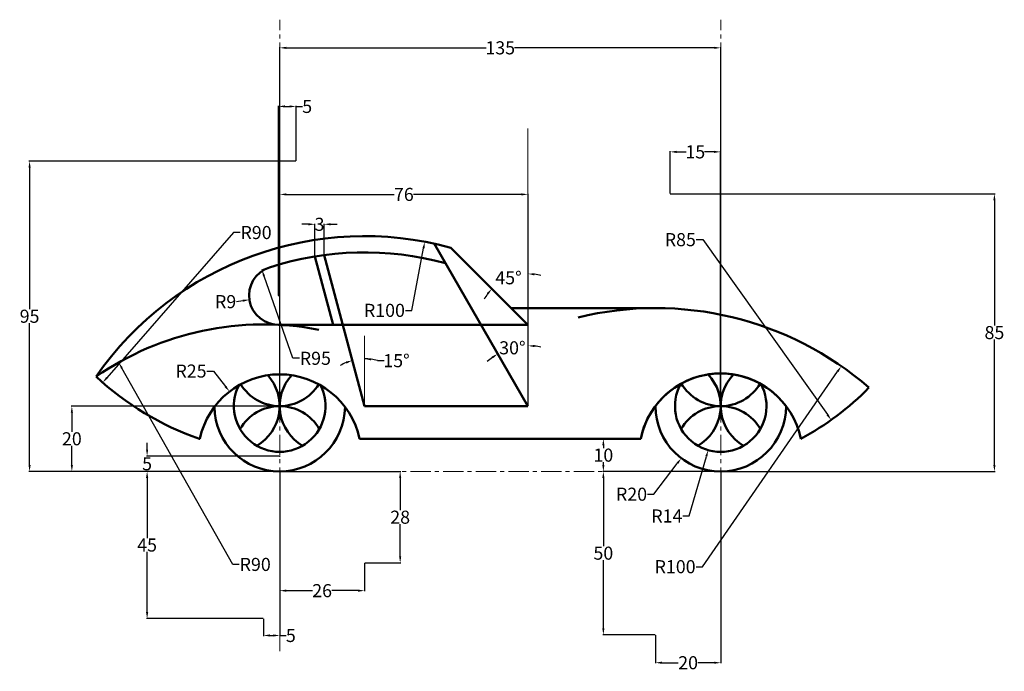
# Model space of a CAD drawing. Units: millimetres. Extents: x -64 to 541, y -54 to 145.
# Tile 1 of 2: x -64 to 238, y -54 to 145. Entities that reach past the tile are written whole.
import ezdxf

# ---------------------------------------------------------------- set-up
doc = ezdxf.new("R2010")
doc.units = ezdxf.units.MM
doc.header["$MEASUREMENT"] = 0
doc.linetypes.add('CENTER', pattern=[2, 1.25, -0.25, 0.25, -0.25])
for name, color, linetype, lineweight in [('M-CNTR', 4, 'CENTER', 18), ('M-CONS', 8, 'Continuous', 13), ('M-DIMS', 2, 'Continuous', 25), ('M-OUTL', 7, 'Continuous', 50)]:
    doc.layers.add(name, color=color, linetype=linetype, lineweight=lineweight)
doc.styles.get("Standard").update_dxf_attribs({"font": 'arial.ttf'})
doc.dimstyles.get("Standard").update_dxf_attribs({"dimtxt": 4, "dimasz": 2, "dimexe": 0.18, "dimexo": 0.0625, "dimgap": 0.09, "dimtad": 0, "dimtih": 1, "dimtoh": 1, "dimdec": 0, "dimzin": 0, "dimdsep": 46, "dimtxsty": 'Standard', "dimcen": 0.09, "dimadec": 0, "dimazin": 0, "dimtfac": 1, "dimtdec": 0, "dimtofl": 0, "dimtmove": 0, "dimatfit": 3, "dimfxl": 1, "dimtolj": 1, "dimtzin": 0, "dimarcsym": 0})

# ---------------------------------------------------------------- blocks, each defined once
blk = doc.blocks.new('*D2')
at = {"layer": 'Defpoints', "color": 0, "transparency": 16777216}
for p in [(15.99, 6.84), (41.96, -21.13), (41.96, -29.63)]:
    blk.add_point(p, dxfattribs=at)
at = {"layer": 'M-DIMS', "color": 0, "lineweight": -2, "transparency": 16777216}
for p, q in [((15.99, 6.78), (15.99, -29.81)), ((41.96, -21.2), (41.96, -29.81)), ((17.99, -29.63), (25.98, -29.63)), ((39.96, -29.63), (31.96, -29.63))]:
    blk.add_line(p, q, dxfattribs=at)
at = {"layer": 'M-DIMS', "color": 0, "transparency": 16777216}
for points in [[(17.99, -29.3), (17.99, -29.97), (15.99, -29.63)], [(39.96, -29.3), (39.96, -29.97), (41.96, -29.63)]]:
    blk.add_solid(points, dxfattribs=at)
at = {"layer": 'M-DIMS', "color": 0, "transparency": 16777216, "insert": (28.97, -29.63), "char_height": 4, "attachment_point": 5}
blk.add_mtext('\\A1;26', dxfattribs=at)
blk = doc.blocks.new('*D3')
at = {"layer": 'Defpoints', "color": 0, "transparency": 16777216}
for p in [(15.99, 6.84), (41.96, -21.13), (52.86, -21.13)]:
    blk.add_point(p, dxfattribs=at)
at = {"layer": 'M-DIMS', "color": 0, "lineweight": -2, "transparency": 16777216}
for p, q in [((16.05, 6.84), (53.04, 6.84)), ((52.86, 4.84), (52.86, -5.02)), ((52.86, -19.13), (52.86, -9.28)), ((42.02, -21.13), (53.04, -21.13))]:
    blk.add_line(p, q, dxfattribs=at)
at = {"layer": 'M-DIMS', "color": 0, "transparency": 16777216}
for points in [[(52.53, 4.84), (53.19, 4.84), (52.86, 6.84)], [(52.53, -19.13), (53.19, -19.13), (52.86, -21.13)]]:
    blk.add_solid(points, dxfattribs=at)
at = {"layer": 'M-DIMS', "color": 0, "transparency": 16777216, "insert": (52.86, -7.15), "char_height": 4, "attachment_point": 5}
blk.add_mtext('\\A1;28', dxfattribs=at)
blk = doc.blocks.new('*D4')
at = {"layer": 'Defpoints', "color": 0, "transparency": 16777216}
for p in [(15.99, 6.84), (10.99, -38.16), (15.99, -43.35)]:
    blk.add_point(p, dxfattribs=at)
at = {"layer": 'M-DIMS', "color": 0, "lineweight": -2, "transparency": 16777216}
for p, q in [((15.99, 6.78), (15.99, -43.53)), ((10.99, -38.22), (10.99, -43.53)), ((12.99, -43.35), (13.99, -43.35)), ((15.99, -43.35), (17.99, -43.35))]:
    blk.add_line(p, q, dxfattribs=at)
at = {"layer": 'M-DIMS', "color": 0, "transparency": 16777216}
for points in [[(12.99, -43.01), (12.99, -43.68), (10.99, -43.35)], [(13.99, -43.01), (13.99, -43.68), (15.99, -43.35)]]:
    blk.add_solid(points, dxfattribs=at)
at = {"layer": 'M-DIMS', "color": 0, "transparency": 16777216, "insert": (19.4, -43.35), "char_height": 4, "attachment_point": 5}
blk.add_mtext('\\A1;5', dxfattribs=at)
blk = doc.blocks.new('*D5')
at = {"layer": 'Defpoints', "color": 0, "transparency": 16777216}
for p in [(-24.6, 6.84), (15.99, 6.84), (10.99, -38.16)]:
    blk.add_point(p, dxfattribs=at)
at = {"layer": 'M-DIMS', "color": 0, "lineweight": -2, "transparency": 16777216}
for p, q in [((15.92, 6.84), (-24.78, 6.84)), ((-24.6, 4.84), (-24.6, -13.54)), ((-24.6, -36.16), (-24.6, -17.79)), ((10.92, -38.16), (-24.78, -38.16))]:
    blk.add_line(p, q, dxfattribs=at)
at = {"layer": 'M-DIMS', "color": 0, "transparency": 16777216}
for points in [[(-24.93, 4.84), (-24.26, 4.84), (-24.6, 6.84)], [(-24.93, -36.16), (-24.26, -36.16), (-24.6, -38.16)]]:
    blk.add_solid(points, dxfattribs=at)
at = {"layer": 'M-DIMS', "color": 0, "transparency": 16777216, "insert": (-24.6, -15.66), "char_height": 4, "attachment_point": 5}
blk.add_mtext('\\A1;45', dxfattribs=at)
blk = doc.blocks.new('*D6')
at = {"layer": 'Defpoints', "color": 0, "transparency": 16777216}
for p in [(-47.63, 26.84), (15.99, 26.84), (15.99, 6.84)]:
    blk.add_point(p, dxfattribs=at)
at = {"layer": 'M-DIMS', "color": 0, "lineweight": -2, "transparency": 16777216}
for p, q in [((15.92, 26.84), (-47.81, 26.84)), ((-47.63, 24.84), (-47.63, 18.97)), ((-47.63, 8.84), (-47.63, 14.71)), ((15.92, 6.84), (-47.81, 6.84))]:
    blk.add_line(p, q, dxfattribs=at)
at = {"layer": 'M-DIMS', "color": 0, "transparency": 16777216}
for points in [[(-47.96, 24.84), (-47.29, 24.84), (-47.63, 26.84)], [(-47.96, 8.84), (-47.29, 8.84), (-47.63, 6.84)]]:
    blk.add_solid(points, dxfattribs=at)
at = {"layer": 'M-DIMS', "color": 0, "transparency": 16777216, "insert": (-47.63, 16.84), "char_height": 4, "attachment_point": 5}
blk.add_mtext('\\A1;20', dxfattribs=at)
blk = doc.blocks.new('*D7')
at = {"layer": 'Defpoints', "color": 0, "transparency": 16777216}
for p in [(-33.29, 40.19), (10.99, -38.16)]:
    blk.add_point(p, dxfattribs=at)
at = {"layer": 'M-DIMS', "color": 0, "lineweight": -2, "transparency": 16777216}
for p, q in [((1.63, -21.6), (-32.31, 38.45)), ((3.63, -21.6), (1.63, -21.6))]:
    blk.add_line(p, q, dxfattribs=at)
at = {"layer": 'M-DIMS', "color": 0, "transparency": 16777216}
blk.add_solid([(-32.02, 38.62), (-32.6, 38.29), (-33.29, 40.19)], dxfattribs=at)
at = {"layer": 'M-DIMS', "color": 0, "transparency": 16777216, "insert": (8.49, -21.6), "char_height": 4, "attachment_point": 5}
blk.add_mtext('\\A1;R90', dxfattribs=at)
blk = doc.blocks.new('*D8')
at = {"layer": 'Defpoints', "color": 0, "transparency": 16777216}
for p in [(0.62, 31.28), (15.99, 11.56)]:
    blk.add_point(p, dxfattribs=at)
at = {"layer": 'M-DIMS', "color": 0, "lineweight": -2, "transparency": 16777216}
for p, q in [((-6.28, 37.57), (-4.28, 37.57)), ((-4.28, 37.57), (-0.61, 32.86)), ((15.9, 11.56), (16.08, 11.56)), ((15.99, 11.47), (15.99, 11.65))]:
    blk.add_line(p, q, dxfattribs=at)
at = {"layer": 'M-DIMS', "color": 0, "transparency": 16777216}
blk.add_solid([(-0.34, 33.06), (-0.87, 32.65), (0.62, 31.28)], dxfattribs=at)
at = {"layer": 'M-DIMS', "color": 0, "transparency": 16777216, "insert": (-11.16, 37.57), "char_height": 4, "attachment_point": 5}
blk.add_mtext('\\A1;R25', dxfattribs=at)
blk = doc.blocks.new('*D9')
at = {"layer": 'Defpoints', "color": 0, "transparency": 16777216}
for p in [(10.54, 68.52), (41.96, -21.13)]:
    blk.add_point(p, dxfattribs=at)
at = {"layer": 'M-DIMS', "color": 0, "lineweight": -2, "transparency": 16777216}
for p, q in [((20.02, 41.47), (11.2, 66.63)), ((22.02, 41.47), (20.02, 41.47))]:
    blk.add_line(p, q, dxfattribs=at)
blk.add_arc((41.96, -21.13), 95, 107.8791, 109.4219, dxfattribs=at)
at = {"layer": 'M-DIMS', "color": 0, "transparency": 16777216}
blk.add_solid([(11.51, 66.74), (10.88, 66.52), (10.54, 68.52)], dxfattribs=at)
at = {"layer": 'M-DIMS', "color": 0, "transparency": 16777216, "insert": (26.9, 41.47), "char_height": 4, "attachment_point": 5}
blk.add_mtext('\\A1;R95', dxfattribs=at)
blk = doc.blocks.new('*D10')
at = {"layer": 'Defpoints', "color": 0, "transparency": 16777216}
for p in [(60.39, 77.15), (41.96, -21.13)]:
    blk.add_point(p, dxfattribs=at)
at = {"layer": 'M-DIMS', "color": 0, "lineweight": -2, "transparency": 16777216}
for p, q in [((56.45, 56.14), (60.02, 75.19)), ((54.45, 56.14), (56.45, 56.14))]:
    blk.add_line(p, q, dxfattribs=at)
at = {"layer": 'M-DIMS', "color": 0, "transparency": 16777216}
blk.add_solid([(59.7, 75.25), (60.35, 75.12), (60.39, 77.15)], dxfattribs=at)
at = {"layer": 'M-DIMS', "color": 0, "transparency": 16777216, "insert": (48.04, 56.14), "char_height": 4, "attachment_point": 5}
blk.add_mtext('\\A1;R100', dxfattribs=at)
blk = doc.blocks.new('*D11')
at = {"layer": 'Defpoints', "color": 0, "transparency": 16777216}
for p in [(20.99, 101.84), (-38.19, 34.03)]:
    blk.add_point(p, dxfattribs=at)
at = {"layer": 'M-DIMS', "color": 0, "lineweight": -2, "transparency": 16777216}
for p, q in [((1.89, 79.95), (-36.88, 35.54)), ((3.89, 79.95), (1.89, 79.95))]:
    blk.add_line(p, q, dxfattribs=at)
at = {"layer": 'M-DIMS', "color": 0, "transparency": 16777216}
blk.add_solid([(-37.13, 35.76), (-36.63, 35.32), (-38.19, 34.03)], dxfattribs=at)
at = {"layer": 'M-DIMS', "color": 0, "transparency": 16777216, "insert": (8.75, 79.95), "char_height": 4, "attachment_point": 5}
blk.add_mtext('\\A1;R90', dxfattribs=at)
blk = doc.blocks.new('*D12')
at = {"layer": 'Defpoints', "color": 0, "transparency": 16777216}
for p in [(91.99, 91.62), (15.99, 26.84), (91.99, 26.84)]:
    blk.add_point(p, dxfattribs=at)
at = {"layer": 'M-DIMS', "color": 0, "lineweight": -2, "transparency": 16777216}
for p, q in [((15.99, 26.9), (15.99, 91.8)), ((17.99, 91.62), (51.05, 91.62)), ((89.99, 91.62), (56.92, 91.62)), ((91.99, 26.9), (91.99, 91.8))]:
    blk.add_line(p, q, dxfattribs=at)
at = {"layer": 'M-DIMS', "color": 0, "transparency": 16777216}
for points in [[(17.99, 91.95), (17.99, 91.29), (15.99, 91.62)], [(89.99, 91.95), (89.99, 91.29), (91.99, 91.62)]]:
    blk.add_solid(points, dxfattribs=at)
at = {"layer": 'M-DIMS', "color": 0, "transparency": 16777216, "insert": (53.99, 91.62), "char_height": 4, "attachment_point": 5}
blk.add_mtext('\\A1;76', dxfattribs=at)
blk = doc.blocks.new('*D13')
at = {"layer": 'Defpoints', "color": 0, "transparency": 16777216}
for p in [(29.57, 82.48), (26.76, 72.64), (29.57, 73.05)]:
    blk.add_point(p, dxfattribs=at)
at = {"layer": 'M-DIMS', "color": 0, "lineweight": -2, "transparency": 16777216}
for p, q in [((24.76, 82.48), (22.76, 82.48)), ((26.76, 72.71), (26.76, 82.66)), ((29.57, 73.12), (29.57, 82.66)), ((31.57, 82.48), (33.57, 82.48))]:
    blk.add_line(p, q, dxfattribs=at)
at = {"layer": 'M-DIMS', "color": 0, "transparency": 16777216}
for points in [[(24.76, 82.82), (24.76, 82.15), (26.76, 82.48)], [(31.57, 82.82), (31.57, 82.15), (29.57, 82.48)]]:
    blk.add_solid(points, dxfattribs=at)
at = {"layer": 'M-DIMS', "color": 0, "transparency": 16777216, "insert": (28.17, 82.48), "char_height": 4, "attachment_point": 5}
blk.add_mtext('\\A1;3', dxfattribs=at)
blk = doc.blocks.new('*D14')
at = {"layer": 'Defpoints', "color": 0, "transparency": 16777216}
for p in [(15.61, 60.73), (6.71, 59.4)]:
    blk.add_point(p, dxfattribs=at)
at = {"layer": 'M-DIMS', "color": 0, "lineweight": -2, "transparency": 16777216}
for p, q in [((15.52, 60.73), (15.7, 60.73)), ((15.61, 60.64), (15.61, 60.82)), ((2.75, 58.81), (4.73, 59.11))]:
    blk.add_line(p, q, dxfattribs=at)
at = {"layer": 'M-DIMS', "color": 0, "transparency": 16777216}
blk.add_solid([(4.68, 59.44), (4.78, 58.78), (6.71, 59.4)], dxfattribs=at)
at = {"layer": 'M-DIMS', "color": 0, "transparency": 16777216, "insert": (-0.57, 58.81), "char_height": 4, "attachment_point": 5}
blk.add_mtext('\\A1;R9', dxfattribs=at)
blk = doc.blocks.new('*D15')
at = {"layer": 'Defpoints', "color": 0, "transparency": 16777216}
for p in [(20.99, 118.54), (20.99, 101.84), (15.61, 60.73)]:
    blk.add_point(p, dxfattribs=at)
at = {"layer": 'M-DIMS', "color": 0, "lineweight": -2, "transparency": 16777216}
for p, q in [((15.61, 60.79), (15.61, 118.72)), ((17.61, 118.54), (18.99, 118.54)), ((20.99, 101.9), (20.99, 118.72)), ((20.99, 118.54), (22.99, 118.54))]:
    blk.add_line(p, q, dxfattribs=at)
at = {"layer": 'M-DIMS', "color": 0, "transparency": 16777216}
for points in [[(17.61, 118.87), (17.61, 118.21), (15.61, 118.54)], [(18.99, 118.87), (18.99, 118.21), (20.99, 118.54)]]:
    blk.add_solid(points, dxfattribs=at)
at = {"layer": 'M-DIMS', "color": 0, "transparency": 16777216, "insert": (24.4, 118.54), "char_height": 4, "attachment_point": 5}
blk.add_mtext('\\A1;5', dxfattribs=at)
blk = doc.blocks.new('*D16')
at = {"layer": 'Defpoints', "color": 0, "transparency": 16777216}
for p in [(-60.57, 101.84), (20.99, 101.84), (15.99, 6.84)]:
    blk.add_point(p, dxfattribs=at)
at = {"layer": 'M-DIMS', "color": 0, "lineweight": -2, "transparency": 16777216}
for p, q in [((20.92, 101.84), (-60.75, 101.84)), ((-60.57, 99.84), (-60.57, 56.47)), ((-60.57, 8.84), (-60.57, 52.21)), ((15.92, 6.84), (-60.75, 6.84))]:
    blk.add_line(p, q, dxfattribs=at)
at = {"layer": 'M-DIMS', "color": 0, "transparency": 16777216}
for points in [[(-60.9, 99.84), (-60.24, 99.84), (-60.57, 101.84)], [(-60.9, 8.84), (-60.24, 8.84), (-60.57, 6.84)]]:
    blk.add_solid(points, dxfattribs=at)
at = {"layer": 'M-DIMS', "color": 0, "transparency": 16777216, "insert": (-60.57, 54.34), "char_height": 4, "attachment_point": 5}
blk.add_mtext('\\A1;95', dxfattribs=at)
blk = doc.blocks.new('*D17')
at = {"layer": 'Defpoints', "color": 0, "transparency": 16777216}
for p in [(150.99, 136.47), (15.99, 26.84), (150.99, 26.84)]:
    blk.add_point(p, dxfattribs=at)
at = {"layer": 'M-DIMS', "color": 0, "lineweight": -2, "transparency": 16777216}
for p, q in [((15.99, 26.9), (15.99, 136.65)), ((17.99, 136.47), (79.15, 136.47)), ((148.99, 136.47), (87.82, 136.47)), ((150.99, 26.9), (150.99, 136.65))]:
    blk.add_line(p, q, dxfattribs=at)
at = {"layer": 'M-DIMS', "color": 0, "transparency": 16777216}
for points in [[(17.99, 136.8), (17.99, 136.14), (15.99, 136.47)], [(148.99, 136.8), (148.99, 136.14), (150.99, 136.47)]]:
    blk.add_solid(points, dxfattribs=at)
at = {"layer": 'M-DIMS', "color": 0, "transparency": 16777216, "insert": (83.49, 136.47), "char_height": 4, "attachment_point": 5}
blk.add_mtext('\\A1;135', dxfattribs=at)
blk = doc.blocks.new('*D18')
at = {"layer": 'Defpoints', "color": 0, "transparency": 16777216}
for p in [(126.49, 16.84), (115.05, 6.84), (150.99, 6.84)]:
    blk.add_point(p, dxfattribs=at)
at = {"layer": 'M-DIMS', "color": 0, "lineweight": -2, "transparency": 16777216}
for p, q in [((126.43, 16.84), (114.87, 16.84)), ((115.05, 14.84), (115.05, 13.97)), ((115.05, 8.84), (115.05, 9.71)), ((150.92, 6.84), (114.87, 6.84))]:
    blk.add_line(p, q, dxfattribs=at)
at = {"layer": 'M-DIMS', "color": 0, "transparency": 16777216}
for points in [[(114.72, 14.84), (115.39, 14.84), (115.05, 16.84)], [(114.72, 8.84), (115.39, 8.84), (115.05, 6.84)]]:
    blk.add_solid(points, dxfattribs=at)
at = {"layer": 'M-DIMS', "color": 0, "transparency": 16777216, "insert": (115.05, 11.84), "char_height": 4, "attachment_point": 5}
blk.add_mtext('\\A1;10', dxfattribs=at)
blk = doc.blocks.new('*D19')
at = {"layer": 'Defpoints', "color": 0, "transparency": 16777216}
for p in [(150.99, 6.84), (115.05, -43.16), (130.99, -43.16)]:
    blk.add_point(p, dxfattribs=at)
at = {"layer": 'M-DIMS', "color": 0, "lineweight": -2, "transparency": 16777216}
for p, q in [((150.92, 6.84), (114.87, 6.84)), ((115.05, 4.84), (115.05, -16.03)), ((115.05, -41.16), (115.05, -20.29)), ((130.92, -43.16), (114.87, -43.16))]:
    blk.add_line(p, q, dxfattribs=at)
at = {"layer": 'M-DIMS', "color": 0, "transparency": 16777216}
for points in [[(114.72, 4.84), (115.39, 4.84), (115.05, 6.84)], [(114.72, -41.16), (115.39, -41.16), (115.05, -43.16)]]:
    blk.add_solid(points, dxfattribs=at)
at = {"layer": 'M-DIMS', "color": 0, "transparency": 16777216, "insert": (115.05, -18.16), "char_height": 4, "attachment_point": 5}
blk.add_mtext('\\A1;50', dxfattribs=at)
blk = doc.blocks.new('*D20')
at = {"layer": 'Defpoints', "color": 0, "transparency": 16777216}
for p in [(150.99, 6.84), (130.99, -43.16), (130.99, -51.69)]:
    blk.add_point(p, dxfattribs=at)
at = {"layer": 'M-DIMS', "color": 0, "lineweight": -2, "transparency": 16777216}
for p, q in [((150.99, 6.78), (150.99, -51.87)), ((130.99, -43.22), (130.99, -51.87)), ((132.99, -51.69), (138, -51.69)), ((148.99, -51.69), (143.97, -51.69))]:
    blk.add_line(p, q, dxfattribs=at)
at = {"layer": 'M-DIMS', "color": 0, "transparency": 16777216}
for points in [[(132.99, -51.35), (132.99, -52.02), (130.99, -51.69)], [(148.99, -51.35), (148.99, -52.02), (150.99, -51.69)]]:
    blk.add_solid(points, dxfattribs=at)
at = {"layer": 'M-DIMS', "color": 0, "transparency": 16777216, "insert": (140.99, -51.69), "char_height": 4, "attachment_point": 5}
blk.add_mtext('\\A1;20', dxfattribs=at)
blk = doc.blocks.new('*D21')
at = {"layer": 'Defpoints', "color": 0, "transparency": 16777216}
for p in [(150.99, 26.84), (138.9, 10.9)]:
    blk.add_point(p, dxfattribs=at)
at = {"layer": 'M-DIMS', "color": 0, "lineweight": -2, "transparency": 16777216}
for p, q in [((150.9, 26.84), (151.08, 26.84)), ((150.99, 26.75), (150.99, 26.93)), ((130.54, -0.12), (137.69, 9.31)), ((128.54, -0.12), (130.54, -0.12))]:
    blk.add_line(p, q, dxfattribs=at)
at = {"layer": 'M-DIMS', "color": 0, "transparency": 16777216}
blk.add_solid([(137.43, 9.51), (137.96, 9.11), (138.9, 10.9)], dxfattribs=at)
at = {"layer": 'M-DIMS', "color": 0, "transparency": 16777216, "insert": (123.68, -0.12), "char_height": 4, "attachment_point": 5}
blk.add_mtext('\\A1;R20', dxfattribs=at)
blk = doc.blocks.new('*D22')
at = {"layer": 'Defpoints', "color": 0, "transparency": 16777216}
for p in [(150.99, 26.84), (147.13, 13.38)]:
    blk.add_point(p, dxfattribs=at)
at = {"layer": 'M-DIMS', "color": 0, "lineweight": -2, "transparency": 16777216}
for p, q in [((150.9, 26.84), (151.08, 26.84)), ((150.99, 26.75), (150.99, 26.93)), ((141.35, -6.78), (146.58, 11.46)), ((139.35, -6.78), (141.35, -6.78))]:
    blk.add_line(p, q, dxfattribs=at)
at = {"layer": 'M-DIMS', "color": 0, "transparency": 16777216}
blk.add_solid([(146.26, 11.55), (146.9, 11.37), (147.13, 13.38)], dxfattribs=at)
at = {"layer": 'M-DIMS', "color": 0, "transparency": 16777216, "insert": (134.49, -6.78), "char_height": 4, "attachment_point": 5}
blk.add_mtext('\\A1;R14', dxfattribs=at)
blk = doc.blocks.new('*D23')
at = {"layer": 'Defpoints', "color": 0, "transparency": 16777216}
for p in [(187.88, 39.07), (130.99, -43.16)]:
    blk.add_point(p, dxfattribs=at)
at = {"layer": 'M-DIMS', "color": 0, "lineweight": -2, "transparency": 16777216}
for p, q in [((145.42, -22.3), (186.74, 37.43)), ((143.42, -22.3), (145.42, -22.3))]:
    blk.add_line(p, q, dxfattribs=at)
at = {"layer": 'M-DIMS', "color": 0, "transparency": 16777216}
blk.add_solid([(186.47, 37.62), (187.02, 37.24), (187.88, 39.07)], dxfattribs=at)
at = {"layer": 'M-DIMS', "color": 0, "transparency": 16777216, "insert": (137.01, -22.3), "char_height": 4, "attachment_point": 5}
blk.add_mtext('\\A1;R100', dxfattribs=at)
blk = doc.blocks.new('*D24')
at = {"layer": 'Defpoints', "color": 0, "transparency": 16777216}
for p in [(135.48, 91.84), (234.75, 91.84), (150.99, 6.84)]:
    blk.add_point(p, dxfattribs=at)
at = {"layer": 'M-DIMS', "color": 0, "lineweight": -2, "transparency": 16777216}
for p, q in [((135.54, 91.84), (234.93, 91.84)), ((234.75, 89.84), (234.75, 51.47)), ((234.75, 8.84), (234.75, 47.21)), ((151.05, 6.84), (234.93, 6.84))]:
    blk.add_line(p, q, dxfattribs=at)
at = {"layer": 'M-DIMS', "color": 0, "transparency": 16777216}
for points in [[(234.42, 89.84), (235.08, 89.84), (234.75, 91.84)], [(234.42, 8.84), (235.08, 8.84), (234.75, 6.84)]]:
    blk.add_solid(points, dxfattribs=at)
at = {"layer": 'M-DIMS', "color": 0, "transparency": 16777216, "insert": (234.75, 49.34), "char_height": 4, "attachment_point": 5}
blk.add_mtext('\\A1;85', dxfattribs=at)
blk = doc.blocks.new('*D25')
at = {"layer": 'Defpoints', "color": 0, "transparency": 16777216}
for p in [(135.48, 104.64), (135.48, 91.84), (150.9, 26.84)]:
    blk.add_point(p, dxfattribs=at)
at = {"layer": 'M-DIMS', "color": 0, "lineweight": -2, "transparency": 16777216}
for p, q in [((135.48, 91.9), (135.48, 104.82)), ((137.48, 104.64), (140.41, 104.64)), ((148.9, 104.64), (145.97, 104.64)), ((150.9, 26.9), (150.9, 104.82))]:
    blk.add_line(p, q, dxfattribs=at)
at = {"layer": 'M-DIMS', "color": 0, "transparency": 16777216}
for points in [[(137.48, 104.97), (137.48, 104.3), (135.48, 104.64)], [(148.9, 104.97), (148.9, 104.3), (150.9, 104.64)]]:
    blk.add_solid(points, dxfattribs=at)
at = {"layer": 'M-DIMS', "color": 0, "transparency": 16777216, "insert": (143.19, 104.64), "char_height": 4, "attachment_point": 5}
blk.add_mtext('\\A1;15', dxfattribs=at)
blk = doc.blocks.new('*D26')
at = {"layer": 'Defpoints', "color": 0, "transparency": 16777216}
for p in [(135.48, 91.84), (184.79, 22.6)]:
    blk.add_point(p, dxfattribs=at)
at = {"layer": 'M-DIMS', "color": 0, "lineweight": -2, "transparency": 16777216}
for p, q in [((143.49, 77.78), (145.49, 77.78)), ((145.49, 77.78), (183.63, 24.23))]:
    blk.add_line(p, q, dxfattribs=at)
at = {"layer": 'M-DIMS', "color": 0, "transparency": 16777216}
blk.add_solid([(183.9, 24.42), (183.35, 24.03), (184.79, 22.6)], dxfattribs=at)
at = {"layer": 'M-DIMS', "color": 0, "transparency": 16777216, "insert": (138.61, 77.78), "char_height": 4, "attachment_point": 5}
blk.add_mtext('\\A1;R85', dxfattribs=at)
blk = doc.blocks.new('*D27')
at = {"layer": 'Defpoints', "color": 0, "transparency": 16777216}
for p in [(-24.6, 11.56), (15.9, 11.56), (15.99, 6.84)]:
    blk.add_point(p, dxfattribs=at)
at = {"layer": 'M-DIMS', "color": 0, "lineweight": -2, "transparency": 16777216}
for p, q in [((-24.6, 13.56), (-24.6, 15.56)), ((15.83, 11.56), (-24.78, 11.56)), ((15.92, 6.84), (-24.78, 6.84)), ((-24.6, 4.84), (-24.6, 2.84))]:
    blk.add_line(p, q, dxfattribs=at)
at = {"layer": 'M-DIMS', "color": 0, "transparency": 16777216}
for points in [[(-24.93, 13.56), (-24.26, 13.56), (-24.6, 11.56)], [(-24.93, 4.84), (-24.26, 4.84), (-24.6, 6.84)]]:
    blk.add_solid(points, dxfattribs=at)
at = {"layer": 'M-DIMS', "color": 0, "transparency": 16777216, "insert": (-24.6, 9.2), "char_height": 4, "attachment_point": 5}
blk.add_mtext('\\A1;5', dxfattribs=at)
blk = doc.blocks.new('*D28')
at = {"layer": 'Defpoints', "color": 0, "transparency": 16777216}
for p in [(91.99, 111.77), (68.37, 75.31), (87.95, 66.77), (91.99, 51.7), (91.99, 26.84)]:
    blk.add_point(p, dxfattribs=at)
at = {"layer": 'M-DIMS', "color": 0, "lineweight": -2, "transparency": 16777216}
for start, end in [(75.302, 82.651), (142.349, 149.698)]:
    blk.add_arc((91.99, 51.7), 15.6, start, end, dxfattribs=at)
at = {"layer": 'M-DIMS', "color": 0, "transparency": 16777216}
for points in [[(93.96, 66.84), (94, 67.51), (91.99, 67.3)], [(79.38, 61.45), (79.88, 61.01), (80.95, 62.73)]]:
    blk.add_solid(points, dxfattribs=at)
at = {"layer": 'M-DIMS', "color": 0, "transparency": 16777216, "insert": (86.02, 66.11), "char_height": 4, "attachment_point": 5}
blk.add_mtext('\\A1;45°', dxfattribs=at)
blk = doc.blocks.new('*D29')
at = {"layer": 'Defpoints', "color": 0, "transparency": 16777216}
for p in [(91.99, 111.77), (63.28, 76.57), (88.78, 45.03), (91.99, 26.84), (91.99, 26.84)]:
    blk.add_point(p, dxfattribs=at)
at = {"layer": 'M-DIMS', "color": 0, "lineweight": -2, "transparency": 16777216}
for start, end in [(77.588, 83.794), (126.206, 132.412)]:
    blk.add_arc((91.99, 26.84), 18.47, start, end, dxfattribs=at)
at = {"layer": 'M-DIMS', "color": 0, "transparency": 16777216}
for points in [[(93.97, 44.87), (94, 45.54), (91.99, 45.31)], [(80.89, 42.02), (81.26, 41.46), (82.75, 42.84)]]:
    blk.add_solid(points, dxfattribs=at)
at = {"layer": 'M-DIMS', "color": 0, "transparency": 16777216, "insert": (87.21, 44.68), "char_height": 4, "attachment_point": 5}
blk.add_mtext('\\A1;30°', dxfattribs=at)
blk = doc.blocks.new('*D30')
at = {"layer": 'Defpoints', "color": 0, "transparency": 16777216}
for p in [(29.57, 73.05), (41.96, 48.32), (39.44, 41.08), (41.96, 26.84), (41.96, 26.84)]:
    blk.add_point(p, dxfattribs=at)
at = {"layer": 'M-DIMS', "color": 0, "lineweight": -2, "transparency": 16777216}
blk.add_line((45.92, 40.75), (47.92, 40.75), dxfattribs=at)
for start, end in [(112.9292, 120.8585), (74.1032, 90), (74.1415, 82.0708)]:
    blk.add_arc((41.96, 26.84), 14.46, start, end, dxfattribs=at)
at = {"layer": 'M-DIMS', "color": 0, "transparency": 16777216}
for points in [[(36.21, 40.47), (36.43, 39.84), (38.21, 40.81)], [(43.93, 40.83), (43.97, 41.5), (41.96, 41.3)]]:
    blk.add_solid(points, dxfattribs=at)
at = {"layer": 'M-DIMS', "color": 0, "transparency": 16777216, "insert": (51.74, 40.75), "char_height": 4, "attachment_point": 5}
blk.add_mtext('\\A1;15°', dxfattribs=at)
blk = doc.blocks.new('SPORTS-CAR-SIDE-PROFILE')
for p, q in [((132.2, 20), (103.49, 69.73)), ((132.2, 44.86), (108.59, 68.48)), ((72.59, 44.86), (66.98, 65.8)), ((82.17, 20), (69.79, 66.22)), ((171.2, 50), (127.07, 50)), ((56.2, 44.86), (132.2, 44.86)), ((82.17, 20), (132.2, 20)), ((31.62, 10), (31.77, 10)), ((80.64, 10), (166.71, 10))]:
    blk.add_line(p, q)
for centre, radius, start, end in [((82.17, -27.97), 100, 74.6835, 145.2591), ((82.17, -27.97), 95, 74.8819, 107.8414), ((55.83, 53.89), 9, 107.8414, 272.4141), ((171.2, -50), 100, 49.1795, 103.6939), ((51.2, -45), 90, 79.1521, 124.6758), ((61.2, 95), 90, 227.1529, 250.8119), ((56.2, 4.72), 25, 12.189, 167.811), ((42.2, 20), 14, 300, 42.4573), ((70.2, 20), 14, 137.5427, 240), ((191.2, 5), 25, 36.8699, 168.463), ((191.2, 5), 25, 11.537, 168.463), ((177.2, 20), 14, 300, 43.8229), ((205.2, 20), 14, 136.1771, 240), ((56.2, 20), 14, 152.7963, 27.2037), ((56.2, 34), 14, 211.4905, 328.5095), ((191.2, 20), 14, 150.9407, 29.0593), ((191.2, 34), 14, 210.4901, 329.5099), ((175.7, 85), 85, 298.0725, 315.739), ((56.2, 20), 20, 180.7904, 359.2096), ((56.2, 6), 14, 30, 150), ((191.2, 20), 20, 180, 0), ((191.2, 6), 14, 30, 150)]:
    blk.add_arc(centre, radius, start, end)

msp = doc.modelspace()

# ---------------------------------------------------------------- linework, layer by layer
at = {"layer": 'M-CNTR', "ltscale": 5}
for p, q in [((15.9864, -48.1676), (15.9864, 145.0833)), ((150.9864, -48.1676), (150.9864, 145.0833)), ((15.9864, 6.8375), (150.9864, 6.8375))]:
    msp.add_line(p, q, dxfattribs=at)
at = {"layer": 'M-CONS'}
for p, q in [((91.9864, 26.8375), (91.9864, 111.7702)), ((41.9562, 26.8375), (41.9562, 48.3205))]:
    msp.add_line(p, q, dxfattribs=at)

# ---------------------------------------------------------------- block references
at = {"layer": 'M-OUTL'}
msp.add_blockref('SPORTS-CAR-SIDE-PROFILE', (-40.218, 6.838), dxfattribs=at)

# ---------------------------------------------------------------- dimensions: what is measured, and where the dimension line sits
at = {"layer": 'M-DIMS'}
for base, p1, p2, picture, middle in [((150.9864, 136.4693), (15.9864, 26.8375), (150.9864, 26.8375), '*D17', (83.4864, 136.4693)), ((20.9864, 118.5405), (15.6073, 60.7296), (20.9864, 101.8375), '*D15', (24.4024, 118.5405)), ((135.4813, 104.6365), (150.8964, 26.8375), (135.4813, 91.8375), '*D25', (143.1888, 104.6365)), ((91.9864, 91.6212), (15.9864, 26.8375), (91.9864, 26.8375), '*D12', (53.9864, 91.6212)), ((29.5723, 82.4849), (26.7642, 72.6429), (29.5723, 73.0549), '*D13', (28.1682, 82.4849)), ((15.9864, -43.3455), (10.9864, -38.1625), (15.9864, 6.8375), '*D4', (19.4024, -43.3455)), ((41.9562, -29.6327), (15.9864, 6.8375), (41.9562, -21.1345), '*D2', (28.9713, -29.6327)), ((130.9864, -51.6855), (150.9864, 6.8375), (130.9864, -43.1625), '*D20', (140.9864, -51.6855))]:
    dim = msp.add_linear_dim(base=base, p1=p1, p2=p2, dimstyle='Standard', override={"dimclrd": 0, "dimclre": 0, "dimclrt": 0}, dxfattribs=at)
    dim.commit()
    dim.dimension.update_dxf_attribs({"geometry": picture, "text_midpoint": middle})
for base, line1, line2, picture, middle in [((88.7785, 45.0305), ((91.9864, 26.8375), (63.2753, 76.5666)), ((91.9864, 26.8375), (91.9864, 111.7702)), '*D29', (87.205, 44.6817)), ((87.9479, 66.7704), ((91.9864, 51.6985), (68.3713, 75.3137)), ((91.9864, 26.8375), (91.9864, 111.7702)), '*D28', (86.0152, 66.1143)), ((39.4447, 41.0811), ((41.9562, 26.8375), (29.5723, 73.0549)), ((41.9562, 26.8375), (41.9562, 48.3205)), '*D30', (51.7431, 40.7477))]:
    dim = msp.add_angular_dim_2l(base=base, line1=line1, line2=line2, dimstyle='Standard', override={"dimclrd": 0, "dimclre": 0, "dimclrt": 0}, dxfattribs=at)
    dim.commit()
    dim.dimension.update_dxf_attribs({"geometry": picture, "text_midpoint": middle})
for base, p1, p2, picture, middle in [((-60.5688, 101.8375), (15.9864, 6.8375), (20.9864, 101.8375), '*D16', (-60.5688, 54.3375)), ((234.7487, 91.8375), (150.9864, 6.8375), (135.4813, 91.8375), '*D24', (234.7487, 49.3375)), ((-47.6277, 26.8375), (15.9864, 6.8375), (15.9864, 26.8375), '*D6', (-47.6277, 16.8375)), ((-24.5955, 11.5591), (15.9864, 6.8375), (15.8964, 11.5591), '*D27', (-24.5955, 9.1983)), ((115.0537, 6.8375), (126.4915, 16.8375), (150.9864, 6.8375), '*D18', (115.0537, 11.8375)), ((-24.5955, 6.8375), (10.9864, -38.1625), (15.9864, 6.8375), '*D5', (-24.5955, -15.6625)), ((52.8599, -21.1345), (15.9864, 6.8375), (41.9562, -21.1345), '*D3', (52.8599, -7.1485)), ((115.0537, -43.1625), (150.9864, 6.8375), (130.9864, -43.1625), '*D19', (115.0537, -18.1625))]:
    dim = msp.add_linear_dim(base=base, p1=p1, p2=p2, angle=90, dimstyle='Standard', override={"dimclrd": 0, "dimclre": 0, "dimclrt": 0}, dxfattribs=at)
    dim.commit()
    dim.dimension.update_dxf_attribs({"geometry": picture, "text_midpoint": middle})
for center, mpoint, picture, middle in [((20.9864, 101.8375), (-38.1915, 34.0291), '*D11', (8.751, 79.9548)), ((135.4813, 91.8375), (184.7851, 22.5979), '*D26', (138.6057, 77.7822)), ((41.9562, -21.1345), (60.3937, 77.1511), '*D10', (48.0353, 56.1354)), ((41.9562, -21.1345), (10.5365, 68.5193), '*D9', (26.9, 41.4701)), ((10.9864, -38.1625), (-33.2906, 40.1928), '*D7', (8.4896, -21.6004)), ((15.9864, 11.5591), (0.6215, 31.2801), '*D8', (-11.1604, 37.5666)), ((130.9864, -43.1625), (187.8829, 39.0737), '*D23', (137.0061, -22.2976)), ((150.9864, 26.8375), (138.9002, 10.9026), '*D21', (123.6794, -0.1179)), ((150.9864, 26.8375), (147.1284, 13.3796), '*D22', (134.4879, -6.7818))]:
    dim = msp.add_radius_dim(center=center, mpoint=mpoint, dimstyle='Standard', override={"dimclrd": 0, "dimclre": 0, "dimclrt": 0}, dxfattribs=at)
    dim.commit()
    dim.dimension.update_dxf_attribs({"geometry": picture, "text_midpoint": middle, "dimtype": 164})
dim = msp.add_radius_dim(center=(15.6073, 60.7296), mpoint=(6.7058, 59.4016), dimstyle='Standard', override={"dimclrd": 0, "dimclre": 0, "dimclrt": 0}, dxfattribs=at)
dim.commit()
dim.dimension.update_dxf_attribs({"geometry": '*D14', "text_midpoint": (-0.5696, 58.8114)})

doc.saveas('drawing.dxf')
